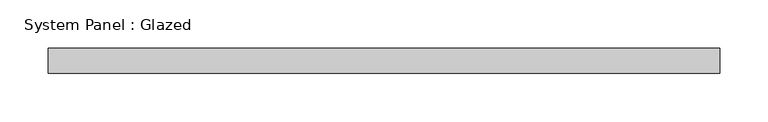
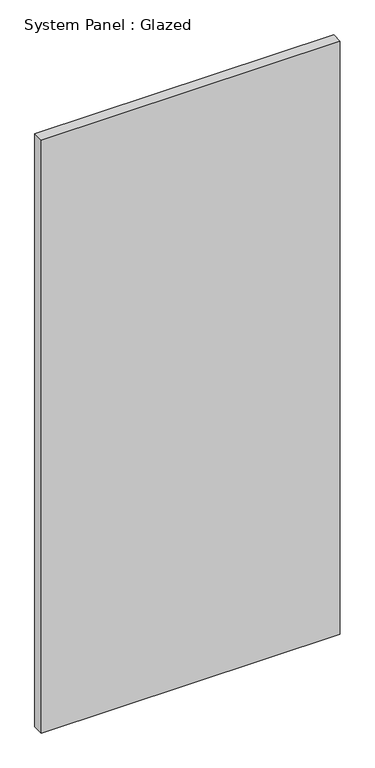
"""IFC4 building model written with IfcOpenShell, lengths in millimetres: plate geometry, System Panel : Glazed."""

from ifc_helpers import new_model, si_unit, origin, origin_with_axes, place, context, project, spatial, polyline, outline, extrude, source, transform, mapped, element, save


def system_panel_glazed_ae4b356e(model_context):
    return source(origin(), model_context, "Body", "SweptSolid", [
        extrude(outline(polyline([(346.075, 19.05), (-346.075, 19.05), (-346.075, 44.45), (346.075, 44.45), (346.075, 19.05)])), origin_with_axes(), (0.0, 0.0, 1.0), 1449.8375758),
    ])


if __name__ == "__main__":
    model = new_model("IFC4")
    model_context = context("Model", 3, world=origin())
    ifc_project = project(units=[si_unit("LENGTHUNIT", "METRE", prefix="MILLI")], contexts=[model_context])
    site = spatial("IfcSite", under=ifc_project)
    building = spatial("IfcBuilding", under=site)
    placement = place(None, origin())
    system_panel_glazed_shape = system_panel_glazed_ae4b356e(model_context)
    element("IfcPlate", 1, ObjectType="System Panel : Glazed", at=placement, inside=building, context=model_context, shape_type="MappedRepresentation", body=[
        mapped(system_panel_glazed_shape, transform((0.0, 0.0, 0.0), x_axis=(1.0, 0.0, 0.0), y_axis=(0.0, 1.0, 0.0), z_axis=(0.0, 0.0, 1.0))),
    ])
    save(model, "model.ifc")

# Revit data of these elements
# Type "System Panel : Glazed"
#   Construction Type Id = "GSP4R"
#   Analytic Construction = "1/8 in Pilkington single glazing"
#   Visual Light Transmittance = 0.9
#   Solar Heat Gain Coefficient = 0.86
#   Heat Transfer Coefficient (U) = 1.18115 BTU/(h·ft²·°F)
#   Define Thermal Properties by = 1
# Element 1 (IfcPlate, "System Panel : Glazed")
#   Materials on its faces: "Glass"
# Materials
#   "Glass": class "Glass", colour RGB 0 128 192, transparency 0.75, Description = "Soda Lime Glass", Cost = 0
